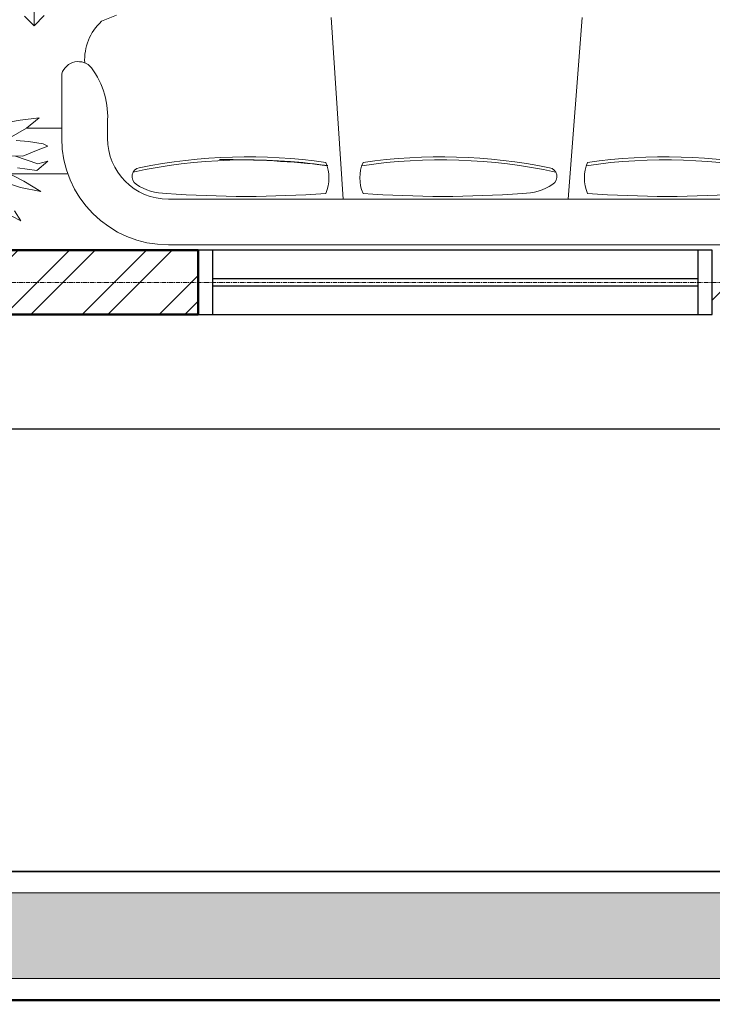
# Model space of a CAD drawing. Units: inches. Extents: x 261 to 2725, y 291 to 1454.
# Tile 9 of 35: x 801 to 898, y 412 to 550. Entities that reach past the tile are written whole.
import ezdxf

# ---------------------------------------------------------------- set-up
doc = ezdxf.new("R2010")
doc.units = ezdxf.units.IN
doc.linetypes.add('CENTER', pattern=[2, 1.25, -0.25, 0.25, -0.25])
for name, color, linetype, lineweight in [('A-ANNO-DIMS', 136, 'Continuous', 18), ('A-FURN', 30, 'Continuous', 18), ('A-GLAZ', 150, 'Continuous', 25), ('A-GRID', 251, 'CENTER', 13), ('A-PLNT', 3, 'Continuous', 18), ('A-PLNT-PATT', 3, 'Continuous', 13), ('A-WALL', 222, 'Continuous', 50), ('A-WALL-PATT', 243, 'Continuous', 13), ('C-PROP', 7, 'Continuous', 35)]:
    doc.layers.add(name, color=color, linetype=linetype, lineweight=lineweight)
doc.styles.get("Standard").update_dxf_attribs({"font": 'arial.ttf'})
doc.dimstyles.new('ISO-25', dxfattribs={"dimtxt": 12, "dimasz": 6, "dimexe": 1.25, "dimexo": 0.625, "dimtad": 1, "dimdec": 0, "dimlunit": 3, "dimtxsty": 'Standard', "dimblk": 'ARCHTICK', "dimcen": 2.5, "dimadec": 0, "dimazin": 0, "dimtfac": 1, "dimtdec": 0, "dimtmove": 0, "dimatfit": 3, "dimfxl": 1, "dimfxlon": 1, "dimarcsym": 0})

# ---------------------------------------------------------------- blocks, each defined once
blk = doc.blocks.new('A$C29956593')
for p, q in [((1017.8, 2786), (2742.6, 2786)), ((2910.7, 2786), (2742.6, 2786)), ((3395.2, 2706.8), (3416.2, 2674.3)), ((3453.6, 2676.8), (3395.2, 2706.8)), ((2910.7, 2636), (1017.8, 2636)), ((1552.3, 2040.1), (1598.4, 2636)), ((2376.2, 2040.1), (2336.4, 2636)), ((3329.8, 2610.4), (3384.7, 2576.6)), ((3396.4, 2597.9), (3329.8, 2610.4)), ((3454.8, 2577.9), (3396.4, 2597.9)), ((3384.7, 2576.6), (3448.9, 2544.1)), ((3431.3, 2553), (3240.6, 2553)), ((3306.4, 2511.5), (3342.6, 2541.6)), ((3342.6, 2541.6), (3405.7, 2532.8)), ((3339.1, 2520.3), (3306.4, 2511.5)), ((3338, 2474), (3388.2, 2495.2)), ((3412.7, 2494.7), (3339.1, 2520.3)), ((3388.2, 2495.2), (3445.4, 2494)), ((3306.4, 2461.5), (3338, 2474)), ((3321.6, 2453.9), (3306.4, 2461.5)), ((3110.7, 2388.1), (3110.7, 2436)), ((3260.7, 2436), (3260.7, 2224.3)), ((3369.5, 2446.4), (3321.6, 2453.9)), ((3410.4, 2443.9), (3369.5, 2446.4)), ((3376.5, 2402.6), (3433.8, 2435.2)), ((3374.8, 2403), (3260.7, 2403)), ((3334.4, 2368.8), (3376.5, 2402.6)), ((3374.8, 2403), (3375.8, 2402)), ((3397.5, 2376.3), (3334.4, 2368.8)), ((3468.8, 2388.9), (3397.5, 2376.3)), ((3130.4, 2052), (3081.5, 2032.1)), ((3351.5, 2067.1), (3317.9, 2033.4)), ((3351.5, 2067.1), (3351.5, 2019.5)), ((3351.5, 2067.1), (3383.5, 2035.1))]:
    blk.add_line(p, q)
for centre, radius, start, end in [((2910.7, 2436), 350, 0, 90), ((1272.9, -801.2), 3428.1, 85.6218, 94.3782), ((2010, -801.2), 3428.1, 85.6218, 94.3782), ((2655.6, -801.2), 3428.1, 85.6218, 94.3782), ((2910.7, 2436), 200, 0, 90), ((1415.2, 2566.2), 129.8, 336.9832, 23.0167), ((1665.5, 2562), 30, 123.4988, 258.5347), ((1748.3, 2436.9), 180, 90, 123.4988), ((2152.3, 2566.2), 129.8, 336.9832, 23.0167), ((2513.3, 2566.2), 129.8, 156.9833, 203.0168), ((2917.3, 2436.9), 180, 56.5012, 90), ((3000.1, 2562), 30, 281.4653, 56.5012), ((1278, 4285.1), 1778.2, 257.8102, 278.4302), ((1278, 4285.1), 1788.2, 258.5347, 278.2533), ((2015, 4285.1), 1778.2, 257.8102, 278.4302), ((2015, 4285.1), 1788.2, 258.5347, 278.2533), ((2735.9, 5677.7), 3171.8, 263.6902, 270.1225), ((2650.6, 4285.1), 1778.2, 261.5698, 282.1898), ((2650.6, 4285.1), 1788.2, 261.7467, 281.4653), ((3381.1, 2366.2), 271.2, 175.359, 216.5496), ((3206.5, 2241.3), 56.8, 220.2227, 342.5272), ((3010.4, 2179.8), 175.3, 313.2134, 2.8934)]:
    blk.add_arc(centre, radius, start, end)
blk = doc.blocks.new('_ArchTick')
at = {"color": 0, "linetype": 'ByBlock', "const_width": 0.15}
blk.add_lwpolyline([(-0.5, -0.5), (0.5, 0.5)], dxfattribs=at)
blk = doc.blocks.new('*D28')
at = {"layer": 'A-ANNO-DIMS', "color": 0, "lineweight": -2, "transparency": 16777216}
for p, q in [((469.45, 349.55), (469.45, 347.3)), ((955.45, 349.55), (955.45, 347.3)), ((469.45, 348.55), (955.45, 348.55))]:
    blk.add_line(p, q, dxfattribs=at)
at = {"layer": 'Defpoints', "color": 0, "transparency": 16777216}
for p in [(469.45, 508.47), (955.45, 508.47), (955.45, 348.55)]:
    blk.add_point(p, dxfattribs=at)
at = {"layer": 'A-ANNO-DIMS', "color": 0, "lineweight": -2, "transparency": 16777216, "xscale": 6, "yscale": 6, "zscale": 6, "rotation": 180}
blk.add_blockref('_ArchTick', (469.45, 348.55), dxfattribs=at)
at = {"layer": 'A-ANNO-DIMS', "color": 0, "lineweight": -2, "transparency": 16777216, "xscale": 6, "yscale": 6, "zscale": 6}
blk.add_blockref('_ArchTick', (955.45, 348.55), dxfattribs=at)
at = {"layer": 'A-ANNO-DIMS', "color": 0, "transparency": 16777216, "insert": (712.45, 355.3), "char_height": 12, "attachment_point": 5}
blk.add_mtext('40\'-6"', dxfattribs=at)
blk = doc.blocks.new('*D31')
at = {"layer": 'A-ANNO-DIMS', "color": 0, "lineweight": -2, "transparency": 16777216}
for p, q in [((478.45, 389.14), (478.45, 386.89)), ((946.45, 389.14), (946.45, 386.89)), ((478.45, 388.14), (946.45, 388.14))]:
    blk.add_line(p, q, dxfattribs=at)
at = {"layer": 'Defpoints', "color": 0, "transparency": 16777216}
for p in [(478.45, 517.47), (946.45, 517.47), (946.45, 388.14)]:
    blk.add_point(p, dxfattribs=at)
at = {"layer": 'A-ANNO-DIMS', "color": 0, "lineweight": -2, "transparency": 16777216, "xscale": 6, "yscale": 6, "zscale": 6, "rotation": 180}
blk.add_blockref('_ArchTick', (478.45, 388.14), dxfattribs=at)
at = {"layer": 'A-ANNO-DIMS', "color": 0, "lineweight": -2, "transparency": 16777216, "xscale": 6, "yscale": 6, "zscale": 6}
blk.add_blockref('_ArchTick', (946.45, 388.14), dxfattribs=at)
at = {"layer": 'A-ANNO-DIMS', "color": 0, "transparency": 16777216, "insert": (712.45, 394.89), "char_height": 12, "attachment_point": 5}
blk.add_mtext("39'", dxfattribs=at)
blk = doc.blocks.new('WIN-72')
for p, q in [((955.45, 950.47), (946.45, 950.47)), ((950.45, 950.47), (950.45, 882.47)), ((951.45, 882.47), (951.45, 950.47)), ((946.45, 882.47), (955.45, 882.47))]:
    blk.add_line(p, q)
blk.add_lwpolyline([(955.45, 880.47), (955.45, 952.47), (946.45, 952.47), (946.45, 880.47)], close=True)
blk = doc.blocks.new('*D67')
at = {"layer": 'A-ANNO-DIMS', "color": 0, "lineweight": -2, "ltscale": 0.07, "transparency": 16777216}
for p, q in [((778.45, 492.4), (526.52, 492.4)), ((778.45, 493.4), (778.45, 491.15)), ((946.45, 492.4), (778.45, 492.4)), ((946.45, 493.4), (946.45, 491.15))]:
    blk.add_line(p, q, dxfattribs=at)
at = {"layer": 'Defpoints', "color": 0, "ltscale": 0.07, "transparency": 16777216}
for p in [(778.45, 517.6), (946.45, 517.6), (778.45, 492.4)]:
    blk.add_point(p, dxfattribs=at)
at = {"layer": 'A-ANNO-DIMS', "color": 0, "lineweight": -2, "ltscale": 0.07, "transparency": 16777216, "xscale": 6, "yscale": 6, "zscale": 6, "rotation": 180}
blk.add_blockref('_ArchTick', (778.45, 492.4), dxfattribs=at)
at = {"layer": 'A-ANNO-DIMS', "color": 0, "lineweight": -2, "ltscale": 0.07, "transparency": 16777216, "xscale": 6, "yscale": 6, "zscale": 6}
blk.add_blockref('_ArchTick', (946.45, 492.4), dxfattribs=at)
at = {"layer": 'A-ANNO-DIMS', "color": 0, "ltscale": 0.07, "transparency": 16777216, "insert": (649.49, 499.24), "char_height": 12, "attachment_point": 5}
blk.add_mtext('LIVING ROOM SOFA SET 14\'-0"', dxfattribs=at)
blk = doc.blocks.new('*D88')
at = {"layer": 'A-ANNO-DIMS', "color": 0, "lineweight": -2, "ltscale": 0.07, "transparency": 16777216}
for p, q in [((430.45, 305.22), (430.45, 302.97)), ((994.45, 305.22), (994.45, 302.97)), ((430.45, 304.22), (994.45, 304.22))]:
    blk.add_line(p, q, dxfattribs=at)
at = {"layer": 'Defpoints', "color": 0, "ltscale": 0.07, "transparency": 16777216}
for p in [(430.45, 412.47), (994.45, 412.47), (994.45, 304.22)]:
    blk.add_point(p, dxfattribs=at)
at = {"layer": 'A-ANNO-DIMS', "color": 0, "lineweight": -2, "ltscale": 0.07, "transparency": 16777216, "xscale": 6, "yscale": 6, "zscale": 6, "rotation": 180}
blk.add_blockref('_ArchTick', (430.45, 304.22), dxfattribs=at)
at = {"layer": 'A-ANNO-DIMS', "color": 0, "lineweight": -2, "ltscale": 0.07, "transparency": 16777216, "xscale": 6, "yscale": 6, "zscale": 6}
blk.add_blockref('_ArchTick', (994.45, 304.22), dxfattribs=at)
at = {"layer": 'A-ANNO-DIMS', "color": 0, "ltscale": 0.07, "transparency": 16777216, "insert": (712.45, 310.97), "char_height": 12, "attachment_point": 5}
blk.add_mtext('47\'-0"', dxfattribs=at)
blk = doc.blocks.new('*D99')
at = {"layer": 'A-ANNO-DIMS', "color": 0, "lineweight": -2, "ltscale": 0.07, "transparency": 16777216}
for p, q in [((825.95, 305.22), (825.95, 302.97)), ((836.95, 305.22), (836.95, 302.97)), ((825.95, 304.22), (836.95, 304.22)), ((836.95, 304.22), (885.42, 304.22))]:
    blk.add_line(p, q, dxfattribs=at)
at = {"layer": 'Defpoints', "color": 0, "ltscale": 0.07, "transparency": 16777216}
for p in [(825.95, 679.47), (836.95, 679.47), (836.95, 304.22)]:
    blk.add_point(p, dxfattribs=at)
at = {"layer": 'A-ANNO-DIMS', "color": 0, "lineweight": -2, "ltscale": 0.07, "transparency": 16777216, "xscale": 6, "yscale": 6, "zscale": 6, "rotation": 180}
blk.add_blockref('_ArchTick', (825.95, 304.22), dxfattribs=at)
at = {"layer": 'A-ANNO-DIMS', "color": 0, "lineweight": -2, "ltscale": 0.07, "transparency": 16777216, "xscale": 6, "yscale": 6, "zscale": 6}
blk.add_blockref('_ArchTick', (836.95, 304.22), dxfattribs=at)
at = {"layer": 'A-ANNO-DIMS', "color": 0, "ltscale": 0.07, "transparency": 16777216, "insert": (864.19, 310.97), "char_height": 12, "attachment_point": 5}
blk.add_mtext('0\'-11"', dxfattribs=at)
blk = doc.blocks.new('*D103')
at = {"layer": 'A-ANNO-DIMS', "color": 0, "lineweight": -2, "ltscale": 0.07, "transparency": 16777216}
for p, q in [((287.06, 1231.47), (284.81, 1231.47)), ((286.06, 439.47), (286.06, 1231.47)), ((287.06, 439.47), (284.81, 439.47))]:
    blk.add_line(p, q, dxfattribs=at)
at = {"layer": 'Defpoints', "color": 0, "ltscale": 0.07, "transparency": 16777216}
for p in [(286.06, 1231.47), (1243.08, 1231.47), (1243.08, 439.47)]:
    blk.add_point(p, dxfattribs=at)
at = {"layer": 'A-ANNO-DIMS', "color": 0, "lineweight": -2, "ltscale": 0.07, "transparency": 16777216, "xscale": 6, "yscale": 6, "zscale": 6}
for p, rotation in [((286.06, 1231.47), 90), ((286.06, 439.47), 270)]:
    blk.add_blockref('_ArchTick', p, dxfattribs=dict(at, rotation=rotation))
at = {"layer": 'A-ANNO-DIMS', "color": 0, "ltscale": 0.07, "transparency": 16777216, "insert": (279.3, 835.47), "char_height": 12, "attachment_point": 5, "rotation": 90}
blk.add_mtext('66\'-0"', dxfattribs=at)
blk = doc.blocks.new('*D106')
at = {"layer": 'A-ANNO-DIMS', "color": 0, "lineweight": -2, "ltscale": 0.07, "transparency": 16777216}
for p, q in [((287.06, 496.47), (284.81, 496.47)), ((286.06, 448.47), (286.06, 496.47)), ((287.06, 448.47), (284.81, 448.47))]:
    blk.add_line(p, q, dxfattribs=at)
at = {"layer": 'Defpoints', "color": 0, "ltscale": 0.07, "transparency": 16777216}
for p in [(286.06, 496.47), (1252.08, 496.47), (1252.08, 448.47)]:
    blk.add_point(p, dxfattribs=at)
at = {"layer": 'A-ANNO-DIMS', "color": 0, "lineweight": -2, "ltscale": 0.07, "transparency": 16777216, "xscale": 6, "yscale": 6, "zscale": 6}
for p, rotation in [((286.06, 496.47), 90), ((286.06, 448.47), 270)]:
    blk.add_blockref('_ArchTick', p, dxfattribs=dict(at, rotation=rotation))
at = {"layer": 'A-ANNO-DIMS', "color": 0, "ltscale": 0.07, "transparency": 16777216, "insert": (279.3, 472.47), "char_height": 12, "attachment_point": 5, "rotation": 90}
blk.add_mtext('4\'-0"', dxfattribs=at)
blk = doc.blocks.new('*D107')
at = {"layer": 'A-ANNO-DIMS', "color": 0, "lineweight": -2, "ltscale": 0.07, "transparency": 16777216}
for p, q in [((287.06, 673.47), (284.81, 673.47)), ((286.06, 496.47), (286.06, 673.47)), ((287.06, 496.47), (284.81, 496.47))]:
    blk.add_line(p, q, dxfattribs=at)
at = {"layer": 'Defpoints', "color": 0, "ltscale": 0.07, "transparency": 16777216}
for p in [(286.06, 673.47), (1252.08, 673.47), (1252.08, 496.47)]:
    blk.add_point(p, dxfattribs=at)
at = {"layer": 'A-ANNO-DIMS', "color": 0, "lineweight": -2, "ltscale": 0.07, "transparency": 16777216, "xscale": 6, "yscale": 6, "zscale": 6}
for p, rotation in [((286.06, 673.47), 90), ((286.06, 496.47), 270)]:
    blk.add_blockref('_ArchTick', p, dxfattribs=dict(at, rotation=rotation))
at = {"layer": 'A-ANNO-DIMS', "color": 0, "ltscale": 0.07, "transparency": 16777216, "insert": (279.3, 584.97), "char_height": 12, "attachment_point": 5, "rotation": 90}
blk.add_mtext('14\'-9"', dxfattribs=at)
blk = doc.blocks.new('*D123')
at = {"layer": 'A-ANNO-DIMS', "color": 0, "lineweight": -2, "ltscale": 0.07, "transparency": 16777216}
for p, q in [((287.06, 1054.85), (284.81, 1054.85)), ((286.06, 439.47), (286.06, 1054.85)), ((287.06, 439.47), (284.81, 439.47))]:
    blk.add_line(p, q, dxfattribs=at)
at = {"layer": 'Defpoints', "color": 0, "ltscale": 0.07, "transparency": 16777216}
for p in [(286.06, 1054.85), (2007.71, 1054.85), (2007.71, 439.47)]:
    blk.add_point(p, dxfattribs=at)
at = {"layer": 'A-ANNO-DIMS', "color": 0, "lineweight": -2, "ltscale": 0.07, "transparency": 16777216, "xscale": 6, "yscale": 6, "zscale": 6}
for p, rotation in [((286.06, 1054.85), 90), ((286.06, 439.47), 270)]:
    blk.add_blockref('_ArchTick', p, dxfattribs=dict(at, rotation=rotation))
at = {"layer": 'A-ANNO-DIMS', "color": 0, "ltscale": 0.07, "transparency": 16777216, "insert": (279.22, 747.16), "char_height": 12, "attachment_point": 5, "rotation": 90}
blk.add_mtext('51\'-3 1/2"', dxfattribs=at)

msp = doc.modelspace()

# ---------------------------------------------------------------- hatches: boundary and pattern name
at = {"layer": 'A-PLNT-PATT'}
h = msp.add_hatch(dxfattribs=at)
h.set_pattern_fill('GRASS', color=256, scale=0.7)
h.paths.add_polyline_path([(658.45, 427.47), (433.45, 427.47), (433.45, 415.47), (658.45, 415.47)])
h.paths.add_polyline_path([(670.45, 421.47), (664.45, 421.47), (664.45, 415.47), (670.45, 415.47)])
h.paths.add_polyline_path([(784.45, 421.47), (778.45, 421.47), (778.45, 415.47), (784.45, 415.47)])
h.paths.add_polyline_path([(991.45, 427.47), (790.45, 427.47), (790.45, 415.47), (991.45, 415.47)])
h.paths.add_polyline_path([(1439.08, 1220.47), (1252.08, 1220.47), (1252.08, 1198.47), (1417.08, 1198.47), (1417.08, 1117.47), (1439.08, 1117.47)])
h.paths.add_polyline_path([(2304.71, 1045.85), (2016.71, 1045.85), (2016.71, 805.87), (2304.71, 805.87)])
h.paths.add_polyline_path([(1267.21, 1201.68), (1431.59, 1201.68), (1431.59, 1218.76), (1267.21, 1218.76)], flags=24)
h.paths.add_polyline_path([(2089.2, 883.04), (2242.64, 883.04), (2242.64, 936.27), (2089.2, 936.27)], flags=24)
at = {"layer": 'A-WALL-PATT'}
h = msp.add_hatch(dxfattribs=at)
h.set_pattern_fill('ANSI32', color=256, scale=0.8)
h.paths.add_polyline_path([(478.45, 685.47), (580.45, 685.47), (580.45, 691.47), (577.45, 691.47), (577.45, 694.47), (571.45, 694.47), (571.45, 691.47), (478.45, 691.47), (478.45, 721.47), (469.45, 721.47), (469.45, 508.47), (538.45, 508.47), (538.45, 517.47), (478.45, 517.47)])
h.paths.add_polyline_path([(694.45, 517.47), (676.45, 517.47), (676.45, 646.47), (670.45, 646.47), (670.45, 517.47), (610.45, 517.47), (610.45, 508.47), (694.45, 508.47)])
h.paths.add_polyline_path([(676.45, 784.47), (478.45, 784.47), (478.45, 844.47), (469.45, 844.47), (469.45, 745.47), (478.45, 745.47), (478.45, 775.47), (571.45, 775.47), (571.45, 724.47), (577.45, 724.47), (577.45, 775.47), (670.45, 775.47), (670.45, 691.47), (610.45, 691.47), (610.45, 685.47), (670.45, 685.47), (670.45, 682.47), (676.45, 682.47)])
h.paths.add_polyline_path([(955.45, 880.47), (946.45, 880.47), (946.45, 808.47), (778.45, 808.47), (778.45, 799.47), (946.45, 799.47), (946.45, 517.47), (898.45, 517.47), (898.45, 508.47), (955.45, 508.47)])
h.paths.add_polyline_path([(778.45, 598.47), (772.45, 598.47), (772.45, 517.47), (754.45, 517.47), (754.45, 508.47), (826.45, 508.47), (826.45, 517.47), (778.45, 517.47)])
h.paths.add_polyline_path([(955.45, 1090.47), (946.45, 1090.47), (946.45, 1030.47), (817.45, 1030.47), (817.45, 1024.47), (946.45, 1024.47), (946.45, 952.47), (955.45, 952.47)])
h.paths.add_polyline_path([(955.45, 1231.47), (730.45, 1231.47), (730.45, 1222.47), (772.45, 1222.47), (772.45, 1096.47), (766.45, 1096.47), (766.45, 1090.47), (772.45, 1090.47), (772.45, 1006.47), (712.45, 1006.47), (712.45, 1000.47), (778.45, 1000.47), (778.45, 1024.47), (781.45, 1024.47), (781.45, 1030.47), (778.45, 1030.47), (778.45, 1222.47), (946.45, 1222.47), (946.45, 1162.47), (955.45, 1162.47)])
h.paths.add_polyline_path([(694.45, 1231.47), (619.45, 1231.47), (619.45, 1222.47), (646.45, 1222.47), (646.45, 1039.47), (652.45, 1039.47), (652.45, 1090.47), (736.45, 1090.47), (736.45, 1096.47), (652.45, 1096.47), (652.45, 1222.47), (694.45, 1222.47)])
h.paths.add_polyline_path([(571.45, 1231.47), (469.45, 1231.47), (469.45, 1099.47), (478.45, 1099.47), (478.45, 1144.47), (544.45, 1144.47), (544.45, 1153.47), (538.45, 1153.47), (538.45, 1150.47), (478.45, 1150.47), (478.45, 1222.47), (538.45, 1222.47), (538.45, 1183.47), (544.45, 1183.47), (544.45, 1222.47), (571.45, 1222.47)])
h.paths.add_polyline_path([(538.45, 1006.47), (478.45, 1006.47), (478.45, 1051.47), (469.45, 1051.47), (469.45, 940.47), (478.45, 940.47), (478.45, 1000.47), (538.45, 1000.47)])
h.paths.add_polyline_path([(652.45, 1006.47), (652.45, 1009.47), (646.45, 1009.47), (646.45, 1006.47), (586.45, 1006.47), (586.45, 1000.47), (652.45, 1000.47)])
h.paths.add_polyline_path([(1288.08, 973.47), (1243.08, 973.47), (1243.08, 920.97), (1252.08, 920.97), (1252.08, 964.47), (1288.08, 964.47)], flags=17)
h.paths.add_polyline_path([(1402.08, 805.47), (1252.08, 805.47), (1252.08, 848.97), (1243.08, 848.97), (1243.08, 757.47), (1252.08, 757.47), (1252.08, 799.47), (1294.08, 799.47), (1372.08, 799.47), (1372.08, 779.47), (1372.08, 715.47), (1378.08, 715.47), (1378.08, 799.47), (1402.08, 799.47)])
h.paths.add_polyline_path([(1252.08, 721.47), (1243.08, 721.47), (1243.08, 439.47), (1729.08, 439.47), (1729.08, 709.47), (1720.08, 709.47), (1720.08, 679.47), (1582.08, 679.47), (1582.08, 670.47), (1588.08, 670.47), (1588.08, 673.47), (1720.08, 673.47), (1720.08, 559.47), (1690.08, 559.47), (1690.08, 550.47), (1720.08, 550.47), (1720.08, 448.47), (1252.08, 448.47), (1252.08, 496.47), (1312.08, 496.47), (1312.08, 505.47), (1252.08, 505.47), (1252.08, 673.47), (1405.08, 673.47), (1405.08, 679.47), (1378.08, 679.47), (1378.08, 685.47), (1372.08, 685.47), (1372.08, 679.47), (1252.08, 679.47)])
h.paths.add_polyline_path([(1450.08, 550.47), (1480.08, 550.47), (1480.08, 559.47), (1450.08, 559.47), (1450.08, 679.47), (1441.08, 679.47), (1441.08, 673.47), (1444.08, 673.47), (1444.08, 505.47), (1384.08, 505.47), (1384.08, 496.47), (1450.08, 496.47)], flags=17)
h.paths.add_polyline_path([(1618.08, 559.47), (1588.08, 559.47), (1588.08, 634.47), (1582.08, 634.47), (1582.08, 559.47), (1552.08, 559.47), (1552.08, 550.47), (1618.08, 550.47)], flags=17)
h.paths.add_polyline_path([(1564.08, 964.47), (1630.08, 964.47), (1630.08, 973.47), (1477.08, 973.47), (1477.08, 964.47), (1558.08, 964.47), (1558.08, 926.22), (1558.08, 887.97), (1486.08, 887.97), (1486.08, 881.97), (1558.08, 881.97), (1558.08, 805.47), (1450.08, 805.47), (1450.08, 845.97), (1444.08, 845.97), (1444.08, 805.47), (1438.08, 805.47), (1438.08, 799.47), (1564.08, 799.47)], flags=17)
h.paths.add_polyline_path([(1453.08, 973.47), (1408.08, 973.47), (1408.08, 964.47), (1444.08, 964.47), (1444.08, 881.97), (1450.08, 881.97), (1456.08, 881.97), (1456.08, 887.97), (1450.08, 887.97), (1450.08, 964.47), (1453.08, 964.47)], flags=17)
h.paths.add_polyline_path([(1729.08, 1231.47), (1243.08, 1231.47), (1243.08, 1167.47), (1252.08, 1167.47), (1252.08, 1222.47), (1441.08, 1222.47), (1441.08, 1045.47), (1648.08, 1045.47), (1648.08, 1051.47), (1450.08, 1051.47), (1450.08, 1074.47), (1450.08, 1222.47), (1472.08, 1222.47), (1720.08, 1222.47), (1720.08, 1051.47), (1708.08, 1051.47), (1708.08, 1045.47), (1720.08, 1045.47), (1720.08, 973.47), (1702.08, 973.47), (1702.08, 964.47), (1720.08, 964.47), (1720.08, 769.47), (1729.08, 769.47)])
h.paths.add_polyline_path([(2493.71, 1054.85), (2007.71, 1054.85), (2007.71, 439.47), (2214.67, 439.47), (2214.67, 496.47), (2493.71, 496.47)])
h.paths.add_polyline_path([(2016.71, 1045.85), (2304.71, 1045.85), (2304.71, 841.47), (2310.71, 841.47), (2310.71, 1045.85), (2484.71, 1045.85), (2484.71, 805.47), (2310.71, 805.47), (2310.71, 811.47), (2304.71, 811.47), (2304.71, 799.47), (2484.71, 799.47), (2484.71, 679.47), (2304.71, 679.47), (2304.71, 673.47), (2484.71, 673.47), (2484.71, 505.47), (2208.67, 505.47), (2208.67, 448.47), (2016.71, 448.47), (2016.71, 799.47), (2304.71, 799.47), (2304.71, 805.47), (2016.71, 805.47)], flags=16)

# ---------------------------------------------------------------- linework, layer by layer
at = {"layer": 'A-GRID', "ltscale": 0.5}
msp.add_line((394.31, 512.97), (1018.31, 512.97), dxfattribs=at)
at = {"layer": 'A-PLNT'}
msp.add_lwpolyline([(790.45, 415.47), (991.45, 415.47), (991.45, 427.47), (790.45, 427.47)], close=True, dxfattribs=at)
at = {"layer": 'A-WALL'}
for p, q in [((778.45, 517.47), (826.45, 517.47)), ((826.45, 517.47), (826.45, 508.47)), ((754.45, 508.47), (826.45, 508.47)), ((430.45, 412.47), (994.45, 412.47))]:
    msp.add_line(p, q, dxfattribs=at)
at = {"layer": 'C-PROP'}
msp.add_lwpolyline([(787.45, 412.47), (994.45, 412.47), (994.45, 430.47), (787.45, 430.47)], close=True, dxfattribs=at)

# ---------------------------------------------------------------- block references
at = {"layer": 'A-FURN', "xscale": 0.0426601237233356, "yscale": 0.0426601237233356, "zscale": 0.0426601237233356, "rotation": 180}
msp.add_blockref('A$C29956593', (946.45, 637.08), dxfattribs=at)
at = {"layer": 'A-GLAZ', "rotation": 269.9999999999998}
msp.add_blockref('WIN-72', (-54.02, 1463.92), dxfattribs=at)

# ---------------------------------------------------------------- dimensions: what is measured, and where the dimension line sits
at = {"layer": 'A-ANNO-DIMS', "ltscale": 0.07}
for base, p1, p2, picture, middle in [((286.06, 1231.47), (1243.08, 439.47), (1243.08, 1231.47), '*D103', (279.3, 835.47)), ((286.06, 1054.85), (2007.71, 439.47), (2007.71, 1054.85), '*D123', (279.22, 747.16)), ((286.06, 673.47), (1252.08, 496.47), (1252.08, 673.47), '*D107', (279.3, 584.97)), ((286.06, 496.47), (1252.08, 448.47), (1252.08, 496.47), '*D106', (279.3, 472.47))]:
    dim = msp.add_linear_dim(base=base, p1=p1, p2=p2, angle=90, dimstyle='ISO-25', override={"dimdec": 1, "dimlfac": 1, "dimrnd": 0, "dimzin": 1, "dimdsep": 46, "dimlunit": 4, "dimfrac": 2}, dxfattribs=at)
    dim.commit()
    dim.dimension.update_dxf_attribs({"geometry": picture, "text_midpoint": middle})
for base, p1, p2, picture, middle in [((836.95, 304.22), (825.95, 679.47), (836.95, 679.47), '*D99', (864.19, 310.97)), ((994.45, 304.22), (430.45, 412.47), (994.45, 412.47), '*D88', (712.45, 310.97))]:
    dim = msp.add_linear_dim(base=base, p1=p1, p2=p2, dimstyle='ISO-25', override={"dimdec": 1, "dimlfac": 1, "dimrnd": 0, "dimzin": 1, "dimdsep": 46, "dimlunit": 4, "dimfrac": 2}, dxfattribs=at)
    dim.commit()
    dim.dimension.update_dxf_attribs({"geometry": picture, "text_midpoint": middle})
dim = msp.add_linear_dim(base=(778.45, 492.4), p1=(946.45, 517.6), p2=(778.45, 517.6), angle=180, text='LIVING ROOM SOFA SET <>', dimstyle='ISO-25', override={"dimdec": 1, "dimrnd": 0, "dimzin": 1, "dimlunit": 4, "dimfrac": 2}, dxfattribs=at)
dim.commit()
dim.dimension.update_dxf_attribs({"geometry": '*D67', "text_midpoint": (649.49, 499.24)})
at = {"layer": 'A-ANNO-DIMS'}
for base, p1, p2, picture, middle in [((946.45, 388.14), (478.45, 517.47), (946.45, 517.47), '*D31', (712.45, 388.14)), ((955.45, 348.55), (469.45, 508.47), (955.45, 508.47), '*D28', (712.45, 348.55))]:
    dim = msp.add_linear_dim(base=base, p1=p1, p2=p2, dimstyle='ISO-25', override={"dimclrd": 0, "dimclre": 0, "dimclrt": 0}, dxfattribs=at)
    dim.commit()
    dim.dimension.update_dxf_attribs({"geometry": picture, "text_midpoint": middle, "dimtype": 160})

doc.saveas('drawing.dxf')
